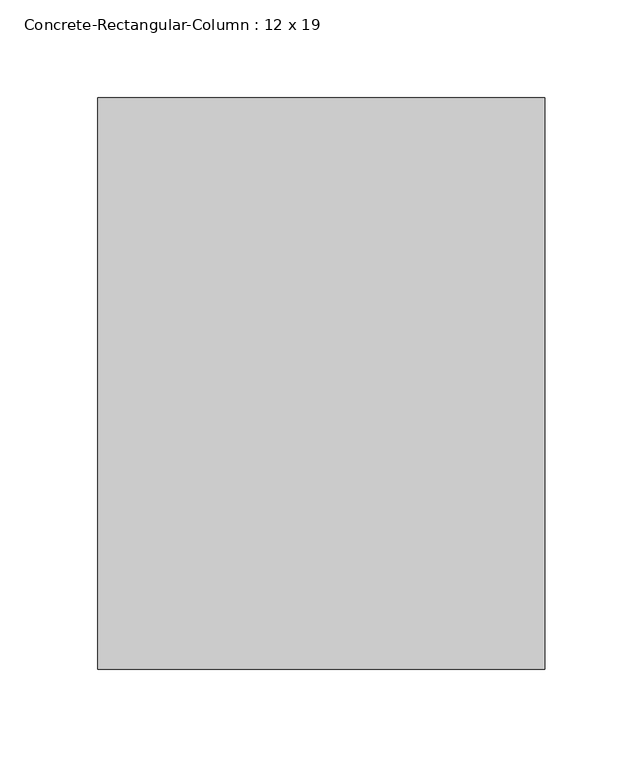
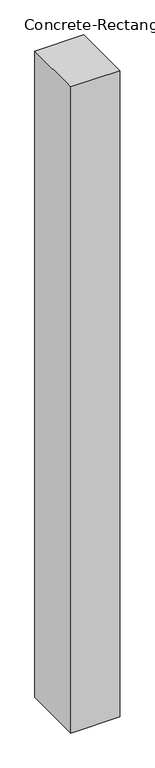
"""IFC4 building model written with IfcOpenShell, lengths in millimetres: column geometry, Concrete-Rectangular-Column : 12 x 19."""

from ifc_helpers import new_model, si_unit, origin, origin_with_axes, place, context, project, spatial, polyline, outline, extrude, source, transform, mapped, element, save


def concrete_rectangular_column_12_x_19_6538d2dd(model_context):
    return source(origin(), model_context, "Body", "SweptSolid", [
        extrude(outline(polyline([(114.3, 146.05), (114.3, -146.05), (-114.3, -146.05), (-114.3, 146.05), (114.3, 146.05)])), origin_with_axes(), (0.0, 0.0, 1.0), 3200.4),
    ])


if __name__ == "__main__":
    model = new_model("IFC4")
    model_context = context("Model", 3, world=origin())
    ifc_project = project(units=[si_unit("LENGTHUNIT", "METRE", prefix="MILLI")], contexts=[model_context])
    site = spatial("IfcSite", under=ifc_project)
    building = spatial("IfcBuilding", under=site)
    placement = place(None, origin())
    concrete_rectangular_column_12_x_19_shape = concrete_rectangular_column_12_x_19_6538d2dd(model_context)
    element("IfcColumn", 1, ObjectType="Concrete-Rectangular-Column : 12 x 19", at=placement, inside=building, context=model_context, shape_type="MappedRepresentation", body=[
        mapped(concrete_rectangular_column_12_x_19_shape, transform((0.0, 0.0, 0.0), x_axis=(1.0, 0.0, 0.0), y_axis=(0.0, 1.0, 0.0), z_axis=(0.0, 0.0, 1.0))),
    ])
    save(model, "model.ifc")

# Revit data of these elements
# Type "Concrete-Rectangular-Column : 12 x 19"
#   Assembly Code = "B10"
#   b = 0' - 9"
#   h = 0' - 11 1/2"
#   Structural Material [instance default] = Concrete, Cast-in-Place gray
# Element 1 (IfcColumn, "Concrete-Rectangular-Column : 12 x 19")
#   Structural Material = Concrete Masonry Units
#   Materials on its faces: "Concrete Masonry Units"
# Materials
#   "Concrete, Cast-in-Place gray": class "Concrete", colour RGB 192 192 192, transparency 0, Description = "Cast-in-place concrete", Cost = 0
#   "Concrete Masonry Units": class "Masonry", colour RGB 63 63 63, transparency 0, Description = "Concrete masonry units", Cost = 0
